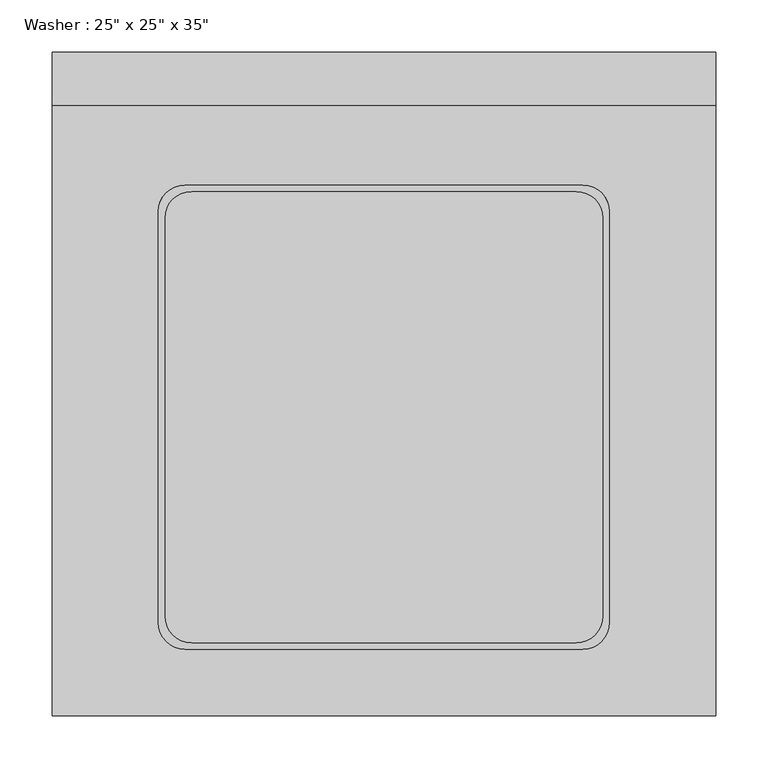
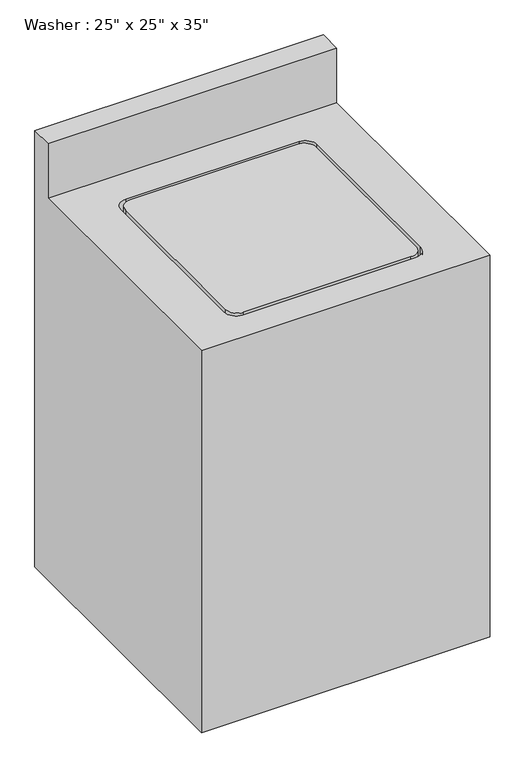
"""IFC4 building model written with IfcOpenShell, lengths in millimetres: proxy geometry."""

from ifc_helpers import new_model, si_unit, point, frame, frame_2d, origin, place, context, project, spatial, polyline, circle_curve, trimmed, segment, composite_curve, outline, extrude, source, transform, mapped, element, save
from ifc_brep_helpers import plane_surface, revolved_surface, advanced_brep


def proxy_1934c8a4(model_context):
    return source(origin(), model_context, "Body", "SolidModel", [
        advanced_brep(
        [(77.5174685, 545.8495648, 889.0), (77.5174685, 545.8495648, 1016.0), (77.5174685, 596.6495648, 1016.0), (77.5174685, 596.6495648, 0.0), (77.5174685, -38.3504352, 0.0), (77.5174685, -38.3504352, 889.0), (712.5174685, 596.6495648, 1016.0), (712.5174685, 545.8495648, 1016.0), (712.5174685, 545.8495648, 889.0), (712.5174685, -38.3504352, 889.0), (712.5174685, -38.3504352, 0.0), (712.5174685, 596.6495648, 0.0), (204.5174685, 469.4681955, 889.0), (585.5174685, 469.4681955, 889.0), (610.9174685, 444.0681955, 889.0), (610.9174685, 50.5495648, 889.0), (585.5174685, 25.1495648, 889.0), (204.5174685, 25.1495648, 889.0), (179.1174685, 50.5495648, 889.0), (179.1174685, 444.0681955, 889.0), (585.5174685, 469.4681955, 838.2), (204.5174685, 469.4681955, 838.2), (179.1174685, 444.0681955, 838.2), (179.1174685, 50.5495648, 838.2), (204.5174685, 25.1495648, 838.2), (585.5174685, 25.1495648, 838.2), (610.9174685, 50.5495648, 838.2), (610.9174685, 444.0681955, 838.2)],
        [
            (0, 1),
            (1, 2),
            (2, 3),
            (3, 4),
            (4, 5),
            (5, 0),
            (6, 7),
            (7, 8),
            (8, 9),
            (9, 10),
            (10, 11),
            (11, 6),
            (0, 8),
            (7, 1),
            (6, 2),
            (11, 3),
            (5, 9),
            (12, 13),
            (13, 14, circle_curve(frame((585.5174685, 444.0681955, 889.0), z_axis=(0.0, 0.0, -1.0), x_axis=(0.0, -1.0, 0.0)), 25.4)),
            (14, 15),
            (15, 16, circle_curve(frame((585.5174685, 50.5495648, 889.0), z_axis=(0.0, 0.0, -1.0), x_axis=(0.0, -1.0, 0.0)), 25.4)),
            (16, 17),
            (17, 18, circle_curve(frame((204.5174685, 50.5495648, 889.0), z_axis=(0.0, 0.0, -1.0), x_axis=(0.0, -1.0, 0.0)), 25.4)),
            (18, 19),
            (19, 12, circle_curve(frame((204.5174685, 444.0681955, 889.0), z_axis=(0.0, 0.0, -1.0), x_axis=(0.0, -1.0, 0.0)), 25.4)),
            (10, 4),
            (20, 21),
            (21, 22, circle_curve(frame((204.5174685, 444.0681955, 838.2), z_axis=(0.0, 0.0, 1.0), x_axis=(0.0, -1.0, 0.0)), 25.4)),
            (22, 23),
            (23, 24, circle_curve(frame((204.5174685, 50.5495648, 838.2), z_axis=(0.0, 0.0, 1.0), x_axis=(0.0, -1.0, 0.0)), 25.4)),
            (24, 25),
            (25, 26, circle_curve(frame((585.5174685, 50.5495648, 838.2), z_axis=(0.0, 0.0, 1.0), x_axis=(0.0, -1.0, 0.0)), 25.4)),
            (26, 27),
            (27, 20, circle_curve(frame((585.5174685, 444.0681955, 838.2), z_axis=(0.0, 0.0, 1.0), x_axis=(0.0, -1.0, 0.0)), 25.4)),
            (20, 13),
            (12, 21),
            (19, 22),
            (18, 23),
            (17, 24),
            (16, 25),
            (15, 26),
            (14, 27),
        ],
        [
            plane_surface(frame((77.5174685, 545.8495648, 889.0), z_axis=(-1.0, 0.0, 0.0), x_axis=(0.0, 0.0, 1.0))),
            plane_surface(frame((712.5174685, 545.8495648, 889.0), z_axis=(1.0, 0.0, 0.0), x_axis=(0.0, 0.0, -1.0))),
            plane_surface(frame((77.5174685, 545.8495648, 889.0), z_axis=(0.0, -1.0, 0.0), x_axis=(1.0, 0.0, 0.0))),
            plane_surface(frame((77.5174685, 545.8495648, 1016.0), z_axis=(0.0, 0.0, 1.0), x_axis=(1.0, 0.0, 0.0))),
            plane_surface(frame((77.5174685, 596.6495648, 1016.0), z_axis=(0.0, 1.0, 0.0), x_axis=(1.0, 0.0, 0.0))),
            plane_surface(frame((77.5174685, -38.3504352, 889.0), z_axis=(0.0, 0.0, 1.0), x_axis=(0.0, -1.0, 0.0))),
            plane_surface(frame((77.5174685, -38.3504352, 0.0), z_axis=(0.0, 0.0, -1.0), x_axis=(0.0, 1.0, 0.0))),
            plane_surface(frame((77.5174685, -38.3504352, 889.0), z_axis=(0.0, -1.0, 0.0), x_axis=(0.0, 0.0, -1.0))),
            plane_surface(frame((204.5174685, 469.4681955, 838.2), z_axis=(0.0, 0.0, 1.0), x_axis=(1.0, 0.0, 0.0))),
            plane_surface(frame((585.5174685, 469.4681955, 889.0), z_axis=(0.0, -1.0, 0.0), x_axis=(0.0, 0.0, -1.0))),
            revolved_surface(polyline([(204.5174685, 418.6681955, 889.0), (204.5174685, 418.6681955, 838.2)]), (204.5174685, 444.0681955, 838.2), (0.0, 0.0, 1.0)),
            plane_surface(frame((179.1174685, 444.0681955, 889.0), z_axis=(1.0, 0.0, 0.0), x_axis=(0.0, 0.0, -1.0))),
            revolved_surface(polyline([(204.5174685, 25.1495648, 889.0), (204.5174685, 25.1495648, 838.2)]), (204.5174685, 50.5495648, 838.2), (0.0, 0.0, 1.0)),
            plane_surface(frame((204.5174685, 25.1495648, 889.0), z_axis=(0.0, 1.0, 0.0), x_axis=(0.0, 0.0, -1.0))),
            revolved_surface(polyline([(585.5174685, 25.1495648, 889.0), (585.5174685, 25.1495648, 838.2)]), (585.5174685, 50.5495648, 838.2), (0.0, 0.0, 1.0)),
            plane_surface(frame((610.9174685, 50.5495648, 889.0), z_axis=(-1.0, 0.0, 0.0), x_axis=(0.0, 0.0, -1.0))),
            revolved_surface(polyline([(585.5174685, 418.6681955, 889.0), (585.5174685, 418.6681955, 838.2)]), (585.5174685, 444.0681955, 838.2), (0.0, 0.0, 1.0)),
        ],
        [
            (0, [[1, 2, 3, 4, 5, 6]]),
            (1, [[7, 8, 9, 10, 11, 12]]),
            (2, [[-1, 13, -8, 14]]),
            (3, [[-2, -14, -7, 15]]),
            (4, [[-15, -12, 16, -3]]),
            (5, [[17, -9, -13, -6], [18, 19, 20, 21, 22, 23, 24, 25]]),
            (6, [[-16, -11, 26, -4]]),
            (7, [[-17, -5, -26, -10]]),
            (8, [[27, 28, 29, 30, 31, 32, 33, 34]]),
            (9, [[-27, 35, -18, 36]]),
            (10, [[-28, -36, -25, 37]]),
            (11, [[-29, -37, -24, 38]]),
            (12, [[-30, -38, -23, 39]]),
            (13, [[-31, -39, -22, 40]]),
            (14, [[-32, -40, -21, 41]]),
            (15, [[-33, -41, -20, 42]]),
            (16, [[-34, -42, -19, -35]]),
        ],
    ),
        extrude(outline(composite_curve([segment(trimmed(circle_curve(frame_2d((210.8674685, 437.8995648)), 25.4), [point((185.4674685, 437.8995648))], [point((210.8674685, 463.2995648))], False, "CARTESIAN"), True, "CONTINUOUS"), segment(polyline([(210.8674685, 463.2995648), (579.1674685, 463.2995648)]), True, "CONTINUOUS"), segment(trimmed(circle_curve(frame_2d((579.1674685, 437.8995648)), 25.4), [point((579.1674685, 463.2995648))], [point((604.5674685, 437.8995648))], False, "CARTESIAN"), True, "CONTINUOUS"), segment(polyline([(604.5674685, 437.8995648), (604.5674685, 56.8995648)]), True, "CONTINUOUS"), segment(trimmed(circle_curve(frame_2d((579.1674685, 56.8995648)), 25.4), [point((604.5674685, 56.8995648))], [point((579.1674685, 31.4995648))], False, "CARTESIAN"), True, "CONTINUOUS"), segment(polyline([(579.1674685, 31.4995648), (210.8674685, 31.4995648)]), True, "CONTINUOUS"), segment(trimmed(circle_curve(frame_2d((210.8674685, 56.8995648)), 25.4), [point((210.8674685, 31.4995648))], [point((185.4674685, 56.8995648))], False, "CARTESIAN"), True, "CONTINUOUS"), segment(polyline([(185.4674685, 56.8995648), (185.4674685, 437.8995648)]), True, "CONTINUOUS")], self_intersect=False)), frame((0.0, 0.0, 863.6), z_axis=(0.0, 0.0, 1.0), x_axis=(1.0, 0.0, 0.0)), (0.0, 0.0, 1.0), 25.4),
    ])


if __name__ == "__main__":
    model = new_model("IFC4")
    model_context = context("Model", 3, world=origin())
    ifc_project = project(units=[si_unit("LENGTHUNIT", "METRE", prefix="MILLI")], contexts=[model_context])
    site = spatial("IfcSite", under=ifc_project)
    building = spatial("IfcBuilding", under=site)
    placement = place(None, origin())
    proxy_shape = proxy_1934c8a4(model_context)
    element("IfcBuildingElementProxy", 1, Name="Washer : 25\" x 25\" x 35\"", ObjectType="Washer : 25\" x 25\" x 35\"", at=placement, inside=building, context=model_context, shape_type="MappedRepresentation", body=[
        mapped(proxy_shape, transform((0.0, 0.0, 0.0), x_axis=(1.0, 0.0, 0.0), y_axis=(0.0, 1.0, 0.0), z_axis=(0.0, 0.0, 1.0))),
    ])
    save(model, "model.ifc")

# Revit data of these elements
# Type "Washer : 25\" x 25\" x 35\""
#   Label = "W"
#   Assembly Code = "E1090400"
#   Depth = 2' - 1"
#   Height = 2' - 11"
#   Width = 2' - 1"
#   Washer Material = Metal - Paint Finish - Ivory,Matte
#   Default Elevation = 0
# Element 1 (IfcBuildingElementProxy, "Washer : 25\" x 25\" x 35\"")
#   Materials on its faces: "Metal - Paint Finish - Ivory,Matte"
# Materials
#   "Metal - Paint Finish - Ivory,Matte": colour RGB 247 247 239, transparency 0
